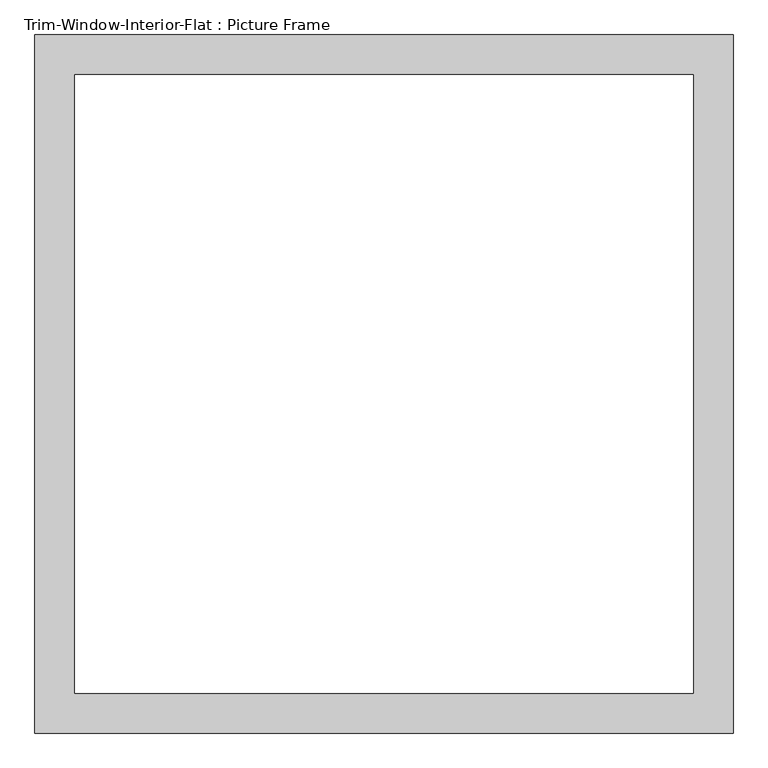
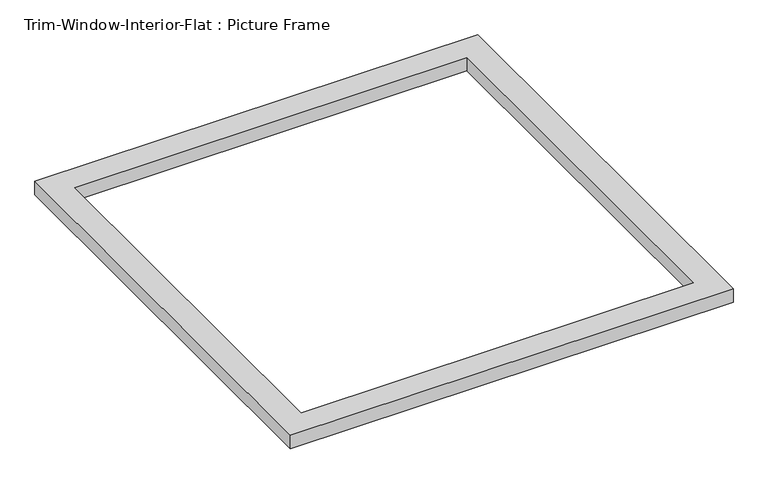
"""IFC4 building model written with IfcOpenShell, lengths in millimetres: proxy geometry, Trim-Window-Interior-Flat : Picture Frame."""

from ifc_helpers import new_model, si_unit, origin, origin_with_axes, place, context, project, spatial, polyline, outline, extrude, source, transform, mapped, element, save


def trim_window_interior_flat_picture_frame_28d4e5dc(model_context):
    return source(origin(), model_context, "Body", "SweptSolid", [
        extrude(outline(polyline([(501.65, 44.45), (501.65, -958.85), (-501.65, -958.85), (-501.65, 44.45), (501.65, 44.45)]), holes=[polyline([(444.5, -12.7), (-444.5, -12.7), (-444.5, -901.7), (444.5, -901.7), (444.5, -12.7)])]), origin_with_axes(), (0.0, 0.0, 1.0), 31.75),
    ])


if __name__ == "__main__":
    model = new_model("IFC4")
    model_context = context("Model", 3, world=origin())
    ifc_project = project(units=[si_unit("LENGTHUNIT", "METRE", prefix="MILLI")], contexts=[model_context])
    site = spatial("IfcSite", under=ifc_project)
    building = spatial("IfcBuilding", under=site)
    placement = place(None, origin())
    trim_window_interior_flat_picture_frame_shape = trim_window_interior_flat_picture_frame_28d4e5dc(model_context)
    element("IfcBuildingElementProxy", 1, Name="Trim-Window-Interior-Flat : Picture Frame", ObjectType="Trim-Window-Interior-Flat : Picture Frame", at=placement, inside=building, context=model_context, shape_type="MappedRepresentation", body=[
        mapped(trim_window_interior_flat_picture_frame_shape, transform((0.0, 0.0, 0.0), x_axis=(1.0, 0.0, 0.0), y_axis=(0.0, 1.0, 0.0), z_axis=(0.0, 0.0, 1.0))),
    ])
    save(model, "model.ifc")

# Revit data of these elements
# Type "Trim-Window-Interior-Flat : Picture Frame"
#   Trim Thickness_Picture Frame = 0' - 1 1/4"
#   Trim Width = 0' - 2 1/4"
#   Trim Thickness_with Sill = 0' - 0 3/4"
#   Sill Thickness = 0' - 1 1/4"
#   Opening Width [instance default] = 2' - 0"
#   Opening Height [instance default] = 3' - 0"
#   Default Elevation = 4' - 0"
#   Sill = no
#   Picture Frame = yes
#   Trim Material [instance default] = none
# Element 1 (IfcBuildingElementProxy, "Trim-Window-Interior-Flat : Picture Frame")
#   Opening Width = 3' - 0"
#   Trim Material = Wood - Stained
#   Materials on its faces: "Wood - Stained"
# Materials
#   "Wood - Stained": class "Wood", colour RGB 224 178 126, transparency 0, Cost = 0
